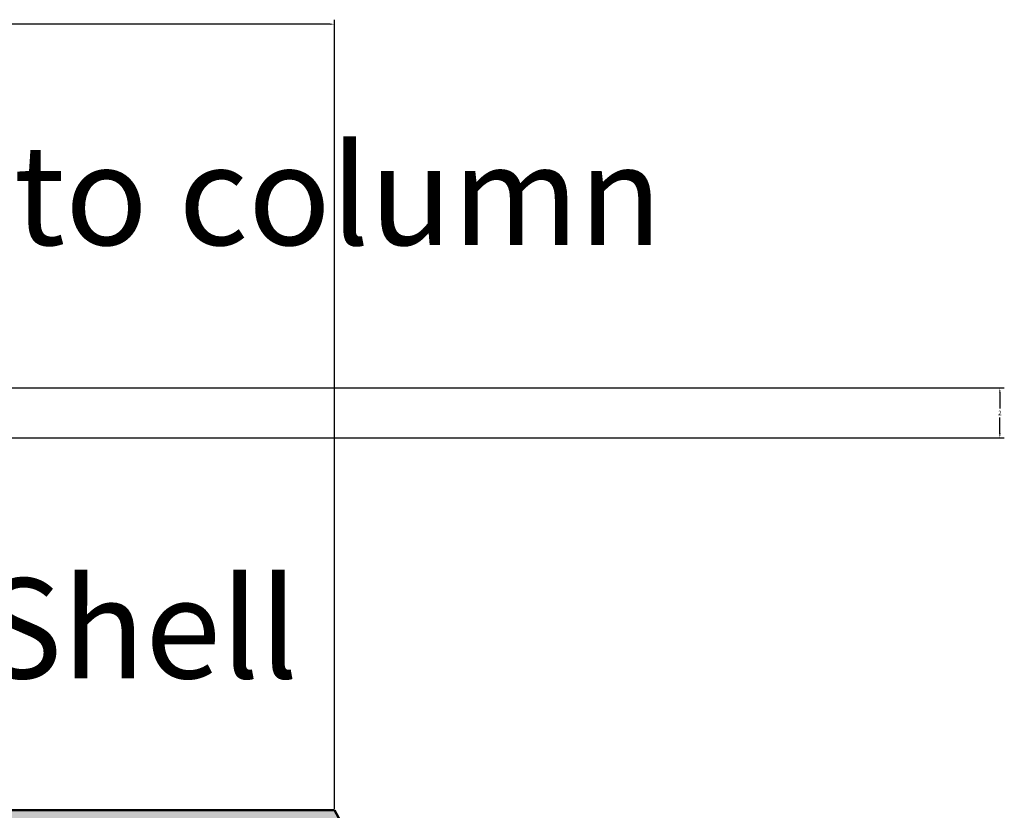
# Model space of a CAD drawing. Units: inches. Extents: x -12 to 334, y -10 to 186.
# Tile 76 of 77: x 257 to 296, y 138 to 170. Entities that reach past the tile are written whole.
import ezdxf
from ezdxf import colors
from ezdxf.entities.mleader import LeaderData, LeaderLine
from ezdxf.math import Vec2, Vec3

# ---------------------------------------------------------------- set-up
doc = ezdxf.new("R2010")
doc.units = ezdxf.units.IN
doc.header["$MEASUREMENT"] = 0
for name, color, linetype, lineweight in [('M-ANNO-TEXT', 3, 'Continuous', 25), ('M-DIMS', 2, 'Continuous', 18), ('M-EQPM', 7, 'Continuous', 50), ('M-EQPM-PATT', 8, 'Continuous', 18)]:
    doc.layers.add(name, color=color, linetype=linetype, lineweight=lineweight)
doc.styles.get("Standard").update_dxf_attribs({"font": 'arial.ttf'})
doc.dimstyles.get("Standard").update_dxf_attribs({"dimtxt": 0.18, "dimasz": 0.18, "dimexe": 0.18, "dimexo": 0.0625, "dimgap": 0.09, "dimtad": 0, "dimtih": 1, "dimtoh": 1, "dimdec": 4, "dimzin": 0, "dimdsep": 46, "dimtxsty": 'Standard', "dimcen": 0.09, "dimadec": 0, "dimazin": 0, "dimtfac": 1, "dimtdec": 4, "dimtofl": 0, "dimtmove": 0, "dimatfit": 3, "dimfxl": 1, "dimtolj": 1, "dimtzin": 0, "dimarcsym": 0})

# ---------------------------------------------------------------- blocks, each defined once
blk = doc.blocks.new('*D21')
at = {"layer": 'Defpoints', "color": 0, "transparency": 16777216}
for p in [(269.381, 169.385), (220.017, 154.835), (269.381, 137.943)]:
    blk.add_point(p, dxfattribs=at)
at = {"layer": 'M-DIMS', "color": 0, "lineweight": -2, "transparency": 16777216}
for p, q in [((220.017, 154.897), (220.017, 169.565)), ((220.197, 169.385), (244.301, 169.385)), ((269.201, 169.385), (245.096, 169.385)), ((269.381, 138.006), (269.381, 169.565))]:
    blk.add_line(p, q, dxfattribs=at)
at = {"layer": 'M-DIMS', "color": 0, "transparency": 16777216}
for points in [[(220.197, 169.415), (220.197, 169.355), (220.017, 169.385)], [(269.201, 169.415), (269.201, 169.355), (269.381, 169.385)]]:
    blk.add_solid(points, dxfattribs=at)
at = {"layer": 'M-DIMS', "color": 0, "transparency": 16777216, "insert": (244.699, 169.385), "char_height": 0.18, "attachment_point": 5}
blk.add_mtext('\\A1;49.36', dxfattribs=at)
blk = doc.blocks.new('*D23')
at = {"layer": 'Defpoints', "color": 0, "transparency": 16777216}
for p in [(220.017, 154.835), (220.017, 152.835), (295.976, 152.835)]:
    blk.add_point(p, dxfattribs=at)
at = {"layer": 'M-DIMS', "color": 0, "lineweight": -2, "transparency": 16777216}
for p, q in [((220.079, 154.835), (296.156, 154.835)), ((295.976, 154.655), (295.976, 154.015)), ((295.976, 153.015), (295.976, 153.654)), ((220.079, 152.835), (296.156, 152.835))]:
    blk.add_line(p, q, dxfattribs=at)
at = {"layer": 'M-DIMS', "color": 0, "transparency": 16777216}
for points in [[(295.946, 154.655), (296.006, 154.655), (295.976, 154.835)], [(295.946, 153.015), (296.006, 153.015), (295.976, 152.835)]]:
    blk.add_solid(points, dxfattribs=at)
at = {"layer": 'M-DIMS', "color": 0, "transparency": 16777216, "insert": (295.976, 153.835), "char_height": 0.18, "attachment_point": 5}
blk.add_mtext('\\A1;2', dxfattribs=at)

msp = doc.modelspace()

# ---------------------------------------------------------------- hatches: boundary and pattern name
at = {"layer": 'M-EQPM-PATT'}
h = msp.add_hatch(color=256, dxfattribs=at)
h.set_gradient(color1=(99, 100, 102), color2=(99, 100, 102), tint=1)
h.paths.add_polyline_path([(126.9567, 136.8871), (179.7818, 136.8871), (180.0106, 137.8871), (126.3793, 137.8871), (106.1771, 102.8958), (86.8879, 102.8958), (86.8879, 109.0583), (84.7229, 109.0583), (84.7229, 100.8958), (106.1771, 100.8958)])
h.paths.add_polyline_path([(196.3421, 152.8345), (195.3421, 152.8345), (195.3421, 137.8871), (180.0106, 137.8871), (179.7818, 136.8871), (196.3421, 136.8871)])
h.paths.add_polyline_path([(215.0166, 152.8345), (214.0166, 152.8345), (214.0166, 136.9435), (268.3808, 136.9435, -0.2673785), (268.3808, 46.8541), (249.3759, 46.8541), (249.8485, 45.8541), (269.3808, 45.8541, 0.2615891), (269.3808, 137.9435), (215.0166, 137.9435)])

# ---------------------------------------------------------------- linework, layer by layer
at = {"layer": 'M-EQPM'}
msp.add_lwpolyline([(215.0166, 152.8345), (215.0166, 137.9435), (269.3808, 137.9435)], dxfattribs=at)
msp.add_arc((187.3936, 91.8988), 94.032, 330.681071, 29.318929, dxfattribs=at)

# ---------------------------------------------------------------- dimensions: what is measured, and where the dimension line sits
at = {"layer": 'M-DIMS'}
dim = msp.add_linear_dim(base=(269.3808, 169.3845), p1=(220.0166, 154.8345), p2=(269.3808, 137.9435), dimstyle='Standard', override={"dimdec": 2, "dimlfac": 1, "dimrnd": 0, "dimzin": 0, "dimdsep": 46, "dimlunit": 2}, dxfattribs=at)
dim.commit()
dim.dimension.update_dxf_attribs({"geometry": '*D21', "text_midpoint": (244.6987, 169.3845)})
dim = msp.add_linear_dim(base=(295.9756, 152.8345), p1=(220.0166, 154.8345), p2=(220.0166, 152.8345), angle=90, dimstyle='Standard', override={"dimdec": 0, "dimlfac": 1, "dimrnd": 0, "dimzin": 0, "dimdsep": 46, "dimlunit": 2}, dxfattribs=at)
dim.commit()
dim.dimension.update_dxf_attribs({"geometry": '*D23', "text_midpoint": (295.9756, 153.8345)})

# ---------------------------------------------------------------- leaders
at = {"layer": 'M-ANNO-TEXT'}
ml = msp.add_multileader_mtext('Standard', dxfattribs=at)
ml.set_content('vapour outlet to column', color=256)
ml.set_leader_properties()
ml.build(insert=Vec2(0, 0))
ml.multileader.update_dxf_attribs({"dogleg_length": 0.36, "arrow_head_size": 0.7})
ctx = ml.context
ctx.base_point, ctx.arrow_head_size, ctx.landing_gap_size, ctx.plane_origin = Vec3(220.6842, 161.9963), 0.7, 0.09, Vec3(211.0929, 154.8345)
notes = []
notes.append((ctx, [(0, (1, 1, 0), (215.2277, 161.9963), (1, 0), 5.4565, [(0, [(211.0929, 154.8345)], 0, [])])]))
ctx.mtext.insert, ctx.mtext.flow_direction = Vec3(220.7742, 164.5515), 5
ml = msp.add_multileader_mtext('Standard', dxfattribs=at)
ml.set_content('Shell', color=256)
ml.set_leader_properties()
ml.build(insert=Vec2(0, 0))
ml.multileader.update_dxf_attribs({"dogleg_length": 0.36, "arrow_head_size": 0.7})
ctx = ml.context
ctx.base_point, ctx.arrow_head_size, ctx.landing_gap_size, ctx.plane_origin = Vec3(255.1635, 145.1886), 0.7, 0.09, Vec3(249.4005, 137.9435)
notes.append((ctx, [(0, (1, 1, 0), (254.8035, 145.1886), (1, 0), 0.36, [(0, [(249.4005, 137.9435)], 0, [])])]))
ctx.mtext.insert, ctx.mtext.flow_direction = Vec3(255.2535, 147.2227), 5
for ctx, leaders in notes:
    for number, flags, end, landing, length, lines in leaders:
        leader = LeaderData()
        leader.index, (leader.has_last_leader_line, leader.has_dogleg_vector, leader.attachment_direction) = number, flags
        leader.last_leader_point, leader.dogleg_vector, leader.dogleg_length = Vec3(end), Vec3(landing), length
        for number, points, colour, breaks in lines:
            line = LeaderLine()
            line.index, line.vertices, line.color, line.breaks = number, Vec3.list(points), colors.encode_raw_color(colour), breaks
            leader.lines.append(line)
        ctx.leaders.append(leader)

doc.saveas('drawing.dxf')
